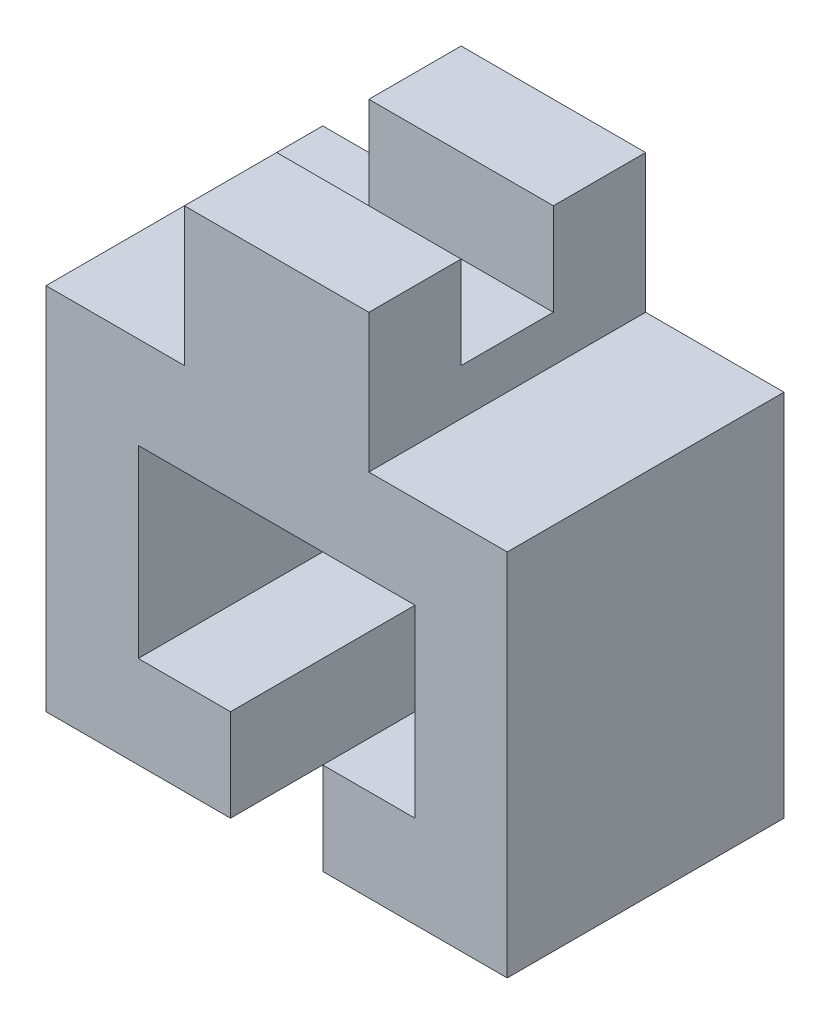
ISO-10303-21;
HEADER;
FILE_DESCRIPTION(('STEP AP214'),'2;1');
FILE_NAME('part.step','',(''),(''),'','','');
FILE_SCHEMA(('AUTOMOTIVE_DESIGN { 1 0 10303 214 1 1 1 1 }'));
ENDSEC;
DATA;
#1=APPLICATION_CONTEXT('core data for automotive mechanical design processes');
#2=APPLICATION_PROTOCOL_DEFINITION('international standard','automotive_design',2000,#1);
#3=PRODUCT_CONTEXT('',#1,'mechanical');
#4=PRODUCT('Part','Part','',(#3));
#5=PRODUCT_RELATED_PRODUCT_CATEGORY('part','',(#4));
#6=PRODUCT_DEFINITION_FORMATION('','',#4);
#7=PRODUCT_DEFINITION_CONTEXT('part definition',#1,'design');
#8=PRODUCT_DEFINITION('design','',#6,#7);
#9=PRODUCT_DEFINITION_SHAPE('','',#8);
#10=(LENGTH_UNIT() NAMED_UNIT(*) SI_UNIT(.MILLI.,.METRE.));
#11=(NAMED_UNIT(*) PLANE_ANGLE_UNIT() SI_UNIT($,.RADIAN.));
#12=(NAMED_UNIT(*) SI_UNIT($,.STERADIAN.) SOLID_ANGLE_UNIT());
#13=UNCERTAINTY_MEASURE_WITH_UNIT(LENGTH_MEASURE(1.E-05),#10,'distance_accuracy_value','');
#14=(GEOMETRIC_REPRESENTATION_CONTEXT(3) GLOBAL_UNCERTAINTY_ASSIGNED_CONTEXT((#13)) GLOBAL_UNIT_ASSIGNED_CONTEXT((#10,
#11,#12)) REPRESENTATION_CONTEXT('',''));
#15=CARTESIAN_POINT('',(0.,0.,0.));
#16=DIRECTION('',(0.,0.,1.));
#17=DIRECTION('',(1.,0.,0.));
#18=AXIS2_PLACEMENT_3D('',#15,#16,#17);
#19=CARTESIAN_POINT('',(15.,55.,30.));
#20=DIRECTION('',(0.,-1.,0.));
#21=DIRECTION('',(0.,0.,-1.));
#22=AXIS2_PLACEMENT_3D('',#19,#20,#21);
#23=PLANE('',#22);
#24=DIRECTION('',(0.,0.,-1.));
#25=VECTOR('',#24,1.);
#26=CARTESIAN_POINT('',(15.,55.,30.));
#27=LINE('',#26,#25);
#28=CARTESIAN_POINT('',(15.,55.,10.));
#29=VERTEX_POINT('',#28);
#30=CARTESIAN_POINT('',(15.,55.,0.));
#31=VERTEX_POINT('',#30);
#32=EDGE_CURVE('E193',#29,#31,#27,.T.);
#33=ORIENTED_EDGE('',*,*,#32,.F.);
#34=DIRECTION('',(-1.,0.,0.));
#35=VECTOR('',#34,1.);
#36=CARTESIAN_POINT('',(15.,55.,10.));
#37=LINE('',#36,#35);
#38=CARTESIAN_POINT('',(35.,55.,10.));
#39=VERTEX_POINT('',#38);
#40=EDGE_CURVE('E346',#39,#29,#37,.T.);
#41=ORIENTED_EDGE('',*,*,#40,.F.);
#42=DIRECTION('',(0.,0.,-1.));
#43=VECTOR('',#42,1.);
#44=CARTESIAN_POINT('',(35.,55.,30.));
#45=LINE('',#44,#43);
#46=CARTESIAN_POINT('',(35.,55.,0.));
#47=VERTEX_POINT('',#46);
#48=EDGE_CURVE('E241',#39,#47,#45,.T.);
#49=ORIENTED_EDGE('',*,*,#48,.T.);
#50=DIRECTION('',(-1.,0.,0.));
#51=VECTOR('',#50,1.);
#52=CARTESIAN_POINT('',(15.,55.,0.));
#53=LINE('',#52,#51);
#54=EDGE_CURVE('E227',#47,#31,#53,.T.);
#55=ORIENTED_EDGE('',*,*,#54,.T.);
#56=EDGE_LOOP('',(#33,#41,#49,#55));
#57=FACE_BOUND('',#56,.T.);
#58=ADVANCED_FACE('F44',(#57),#23,.F.);
#59=CARTESIAN_POINT('',(20.,0.,30.));
#60=DIRECTION('',(0.,1.,0.));
#61=DIRECTION('',(0.,0.,1.));
#62=AXIS2_PLACEMENT_3D('',#59,#60,#61);
#63=PLANE('',#62);
#64=DIRECTION('',(1.,0.,0.));
#65=VECTOR('',#64,1.);
#66=CARTESIAN_POINT('',(20.,0.,0.));
#67=LINE('',#66,#65);
#68=CARTESIAN_POINT('',(0.,0.,0.));
#69=VERTEX_POINT('',#68);
#70=CARTESIAN_POINT('',(20.,0.,0.));
#71=VERTEX_POINT('',#70);
#72=EDGE_CURVE('E201',#69,#71,#67,.T.);
#73=ORIENTED_EDGE('',*,*,#72,.T.);
#74=DIRECTION('',(0.,0.,-1.));
#75=VECTOR('',#74,1.);
#76=CARTESIAN_POINT('',(20.,0.,30.));
#77=LINE('',#76,#75);
#78=CARTESIAN_POINT('',(20.,0.,30.));
#79=VERTEX_POINT('',#78);
#80=EDGE_CURVE('E11',#79,#71,#77,.T.);
#81=ORIENTED_EDGE('',*,*,#80,.F.);
#82=DIRECTION('',(1.,0.,0.));
#83=VECTOR('',#82,1.);
#84=CARTESIAN_POINT('',(20.,0.,30.));
#85=LINE('',#84,#83);
#86=CARTESIAN_POINT('',(0.,0.,30.));
#87=VERTEX_POINT('',#86);
#88=EDGE_CURVE('E240',#87,#79,#85,.T.);
#89=ORIENTED_EDGE('',*,*,#88,.F.);
#90=DIRECTION('',(0.,0.,-1.));
#91=VECTOR('',#90,1.);
#92=CARTESIAN_POINT('',(0.,0.,30.));
#93=LINE('',#92,#91);
#94=EDGE_CURVE('E200',#87,#69,#93,.T.);
#95=ORIENTED_EDGE('',*,*,#94,.T.);
#96=EDGE_LOOP('',(#73,#81,#89,#95));
#97=FACE_BOUND('',#96,.T.);
#98=ADVANCED_FACE('F50',(#97),#63,.F.);
#99=CARTESIAN_POINT('',(20.,10.,30.));
#100=DIRECTION('',(-1.,0.,0.));
#101=DIRECTION('',(0.,0.,1.));
#102=AXIS2_PLACEMENT_3D('',#99,#100,#101);
#103=PLANE('',#102);
#104=DIRECTION('',(0.,1.,0.));
#105=VECTOR('',#104,1.);
#106=CARTESIAN_POINT('',(20.,10.,0.));
#107=LINE('',#106,#105);
#108=CARTESIAN_POINT('',(20.,10.,0.));
#109=VERTEX_POINT('',#108);
#110=EDGE_CURVE('E206',#71,#109,#107,.T.);
#111=ORIENTED_EDGE('',*,*,#110,.T.);
#112=DIRECTION('',(0.,0.,-1.));
#113=VECTOR('',#112,1.);
#114=CARTESIAN_POINT('',(20.,10.,30.));
#115=LINE('',#114,#113);
#116=CARTESIAN_POINT('',(20.,10.,30.));
#117=VERTEX_POINT('',#116);
#118=EDGE_CURVE('E52',#117,#109,#115,.T.);
#119=ORIENTED_EDGE('',*,*,#118,.F.);
#120=DIRECTION('',(0.,1.,0.));
#121=VECTOR('',#120,1.);
#122=CARTESIAN_POINT('',(20.,10.,30.));
#123=LINE('',#122,#121);
#124=EDGE_CURVE('E133',#79,#117,#123,.T.);
#125=ORIENTED_EDGE('',*,*,#124,.F.);
#126=ORIENTED_EDGE('',*,*,#80,.T.);
#127=EDGE_LOOP('',(#111,#119,#125,#126));
#128=FACE_BOUND('',#127,.T.);
#129=ADVANCED_FACE('F369',(#128),#103,.F.);
#130=CARTESIAN_POINT('',(9.99999999999999,10.,30.));
#131=DIRECTION('',(0.,-1.,0.));
#132=DIRECTION('',(0.,0.,-1.));
#133=AXIS2_PLACEMENT_3D('',#130,#131,#132);
#134=PLANE('',#133);
#135=DIRECTION('',(-1.,0.,0.));
#136=VECTOR('',#135,1.);
#137=CARTESIAN_POINT('',(9.99999999999999,10.,0.));
#138=LINE('',#137,#136);
#139=CARTESIAN_POINT('',(9.99999999999999,10.,0.));
#140=VERTEX_POINT('',#139);
#141=EDGE_CURVE('E207',#109,#140,#138,.T.);
#142=ORIENTED_EDGE('',*,*,#141,.T.);
#143=DIRECTION('',(0.,0.,-1.));
#144=VECTOR('',#143,1.);
#145=CARTESIAN_POINT('',(9.99999999999999,10.,30.));
#146=LINE('',#145,#144);
#147=CARTESIAN_POINT('',(9.99999999999999,10.,30.));
#148=VERTEX_POINT('',#147);
#149=EDGE_CURVE('E269',#148,#140,#146,.T.);
#150=ORIENTED_EDGE('',*,*,#149,.F.);
#151=DIRECTION('',(-1.,0.,0.));
#152=VECTOR('',#151,1.);
#153=CARTESIAN_POINT('',(9.99999999999999,10.,30.));
#154=LINE('',#153,#152);
#155=EDGE_CURVE('E279',#117,#148,#154,.T.);
#156=ORIENTED_EDGE('',*,*,#155,.F.);
#157=ORIENTED_EDGE('',*,*,#118,.T.);
#158=EDGE_LOOP('',(#142,#150,#156,#157));
#159=FACE_BOUND('',#158,.T.);
#160=ADVANCED_FACE('F277',(#159),#134,.F.);
#161=CARTESIAN_POINT('',(9.99999999999999,30.,30.));
#162=DIRECTION('',(-1.,0.,0.));
#163=DIRECTION('',(0.,0.,1.));
#164=AXIS2_PLACEMENT_3D('',#161,#162,#163);
#165=PLANE('',#164);
#166=DIRECTION('',(0.,1.,0.));
#167=VECTOR('',#166,1.);
#168=CARTESIAN_POINT('',(9.99999999999999,30.,0.));
#169=LINE('',#168,#167);
#170=CARTESIAN_POINT('',(9.99999999999999,30.,0.));
#171=VERTEX_POINT('',#170);
#172=EDGE_CURVE('E211',#140,#171,#169,.T.);
#173=ORIENTED_EDGE('',*,*,#172,.T.);
#174=DIRECTION('',(0.,0.,-1.));
#175=VECTOR('',#174,1.);
#176=CARTESIAN_POINT('',(9.99999999999999,30.,30.));
#177=LINE('',#176,#175);
#178=CARTESIAN_POINT('',(9.99999999999999,30.,30.));
#179=VERTEX_POINT('',#178);
#180=EDGE_CURVE('E270',#179,#171,#177,.T.);
#181=ORIENTED_EDGE('',*,*,#180,.F.);
#182=DIRECTION('',(0.,1.,0.));
#183=VECTOR('',#182,1.);
#184=CARTESIAN_POINT('',(9.99999999999999,30.,30.));
#185=LINE('',#184,#183);
#186=EDGE_CURVE('E299',#148,#179,#185,.T.);
#187=ORIENTED_EDGE('',*,*,#186,.F.);
#188=ORIENTED_EDGE('',*,*,#149,.T.);
#189=EDGE_LOOP('',(#173,#181,#187,#188));
#190=FACE_BOUND('',#189,.T.);
#191=ADVANCED_FACE('F286',(#190),#165,.F.);
#192=CARTESIAN_POINT('',(40.,30.,30.));
#193=DIRECTION('',(0.,1.,0.));
#194=DIRECTION('',(0.,0.,1.));
#195=AXIS2_PLACEMENT_3D('',#192,#193,#194);
#196=PLANE('',#195);
#197=DIRECTION('',(1.,0.,0.));
#198=VECTOR('',#197,1.);
#199=CARTESIAN_POINT('',(40.,30.,0.));
#200=LINE('',#199,#198);
#201=CARTESIAN_POINT('',(40.,30.,0.));
#202=VERTEX_POINT('',#201);
#203=EDGE_CURVE('E213',#171,#202,#200,.T.);
#204=ORIENTED_EDGE('',*,*,#203,.T.);
#205=DIRECTION('',(0.,0.,-1.));
#206=VECTOR('',#205,1.);
#207=CARTESIAN_POINT('',(40.,30.,30.));
#208=LINE('',#207,#206);
#209=CARTESIAN_POINT('',(40.,30.,30.));
#210=VERTEX_POINT('',#209);
#211=EDGE_CURVE('E262',#210,#202,#208,.T.);
#212=ORIENTED_EDGE('',*,*,#211,.F.);
#213=DIRECTION('',(1.,0.,0.));
#214=VECTOR('',#213,1.);
#215=CARTESIAN_POINT('',(40.,30.,30.));
#216=LINE('',#215,#214);
#217=EDGE_CURVE('E291',#179,#210,#216,.T.);
#218=ORIENTED_EDGE('',*,*,#217,.F.);
#219=ORIENTED_EDGE('',*,*,#180,.T.);
#220=EDGE_LOOP('',(#204,#212,#218,#219));
#221=FACE_BOUND('',#220,.T.);
#222=ADVANCED_FACE('F292',(#221),#196,.F.);
#223=CARTESIAN_POINT('',(40.,10.,30.));
#224=DIRECTION('',(1.,0.,0.));
#225=DIRECTION('',(0.,0.,-1.));
#226=AXIS2_PLACEMENT_3D('',#223,#224,#225);
#227=PLANE('',#226);
#228=DIRECTION('',(0.,-1.,0.));
#229=VECTOR('',#228,1.);
#230=CARTESIAN_POINT('',(40.,10.,0.));
#231=LINE('',#230,#229);
#232=CARTESIAN_POINT('',(40.,10.,0.));
#233=VERTEX_POINT('',#232);
#234=EDGE_CURVE('E214',#202,#233,#231,.T.);
#235=ORIENTED_EDGE('',*,*,#234,.T.);
#236=DIRECTION('',(0.,0.,-1.));
#237=VECTOR('',#236,1.);
#238=CARTESIAN_POINT('',(40.,10.,30.));
#239=LINE('',#238,#237);
#240=CARTESIAN_POINT('',(40.,10.,30.));
#241=VERTEX_POINT('',#240);
#242=EDGE_CURVE('E261',#241,#233,#239,.T.);
#243=ORIENTED_EDGE('',*,*,#242,.F.);
#244=DIRECTION('',(0.,-1.,0.));
#245=VECTOR('',#244,1.);
#246=CARTESIAN_POINT('',(40.,10.,30.));
#247=LINE('',#246,#245);
#248=EDGE_CURVE('E293',#210,#241,#247,.T.);
#249=ORIENTED_EDGE('',*,*,#248,.F.);
#250=ORIENTED_EDGE('',*,*,#211,.T.);
#251=EDGE_LOOP('',(#235,#243,#249,#250));
#252=FACE_BOUND('',#251,.T.);
#253=ADVANCED_FACE('F414',(#252),#227,.F.);
#254=CARTESIAN_POINT('',(30.,10.,30.));
#255=DIRECTION('',(0.,-1.,0.));
#256=DIRECTION('',(0.,0.,-1.));
#257=AXIS2_PLACEMENT_3D('',#254,#255,#256);
#258=PLANE('',#257);
#259=DIRECTION('',(-1.,0.,0.));
#260=VECTOR('',#259,1.);
#261=CARTESIAN_POINT('',(30.,10.,0.));
#262=LINE('',#261,#260);
#263=CARTESIAN_POINT('',(30.,10.,0.));
#264=VERTEX_POINT('',#263);
#265=EDGE_CURVE('E220',#233,#264,#262,.T.);
#266=ORIENTED_EDGE('',*,*,#265,.T.);
#267=DIRECTION('',(0.,0.,-1.));
#268=VECTOR('',#267,1.);
#269=CARTESIAN_POINT('',(30.,10.,30.));
#270=LINE('',#269,#268);
#271=CARTESIAN_POINT('',(30.,10.,30.));
#272=VERTEX_POINT('',#271);
#273=EDGE_CURVE('E256',#272,#264,#270,.T.);
#274=ORIENTED_EDGE('',*,*,#273,.F.);
#275=DIRECTION('',(-1.,0.,0.));
#276=VECTOR('',#275,1.);
#277=CARTESIAN_POINT('',(30.,10.,30.));
#278=LINE('',#277,#276);
#279=EDGE_CURVE('E300',#241,#272,#278,.T.);
#280=ORIENTED_EDGE('',*,*,#279,.F.);
#281=ORIENTED_EDGE('',*,*,#242,.T.);
#282=EDGE_LOOP('',(#266,#274,#280,#281));
#283=FACE_BOUND('',#282,.T.);
#284=ADVANCED_FACE('F406',(#283),#258,.F.);
#285=CARTESIAN_POINT('',(30.,0.,30.));
#286=DIRECTION('',(1.,0.,0.));
#287=DIRECTION('',(0.,0.,-1.));
#288=AXIS2_PLACEMENT_3D('',#285,#286,#287);
#289=PLANE('',#288);
#290=DIRECTION('',(0.,-1.,0.));
#291=VECTOR('',#290,1.);
#292=CARTESIAN_POINT('',(30.,0.,0.));
#293=LINE('',#292,#291);
#294=CARTESIAN_POINT('',(30.,0.,0.));
#295=VERTEX_POINT('',#294);
#296=EDGE_CURVE('E218',#264,#295,#293,.T.);
#297=ORIENTED_EDGE('',*,*,#296,.T.);
#298=DIRECTION('',(0.,0.,-1.));
#299=VECTOR('',#298,1.);
#300=CARTESIAN_POINT('',(30.,0.,30.));
#301=LINE('',#300,#299);
#302=CARTESIAN_POINT('',(30.,0.,30.));
#303=VERTEX_POINT('',#302);
#304=EDGE_CURVE('E254',#303,#295,#301,.T.);
#305=ORIENTED_EDGE('',*,*,#304,.F.);
#306=DIRECTION('',(0.,-1.,0.));
#307=VECTOR('',#306,1.);
#308=CARTESIAN_POINT('',(30.,0.,30.));
#309=LINE('',#308,#307);
#310=EDGE_CURVE('E303',#272,#303,#309,.T.);
#311=ORIENTED_EDGE('',*,*,#310,.F.);
#312=ORIENTED_EDGE('',*,*,#273,.T.);
#313=EDGE_LOOP('',(#297,#305,#311,#312));
#314=FACE_BOUND('',#313,.T.);
#315=ADVANCED_FACE('F401',(#314),#289,.F.);
#316=CARTESIAN_POINT('',(50.,0.,30.));
#317=DIRECTION('',(0.,1.,0.));
#318=DIRECTION('',(0.,0.,1.));
#319=AXIS2_PLACEMENT_3D('',#316,#317,#318);
#320=PLANE('',#319);
#321=DIRECTION('',(1.,0.,0.));
#322=VECTOR('',#321,1.);
#323=CARTESIAN_POINT('',(50.,0.,0.));
#324=LINE('',#323,#322);
#325=CARTESIAN_POINT('',(50.,0.,0.));
#326=VERTEX_POINT('',#325);
#327=EDGE_CURVE('E222',#295,#326,#324,.T.);
#328=ORIENTED_EDGE('',*,*,#327,.T.);
#329=DIRECTION('',(0.,0.,-1.));
#330=VECTOR('',#329,1.);
#331=CARTESIAN_POINT('',(50.,0.,30.));
#332=LINE('',#331,#330);
#333=CARTESIAN_POINT('',(50.,0.,30.));
#334=VERTEX_POINT('',#333);
#335=EDGE_CURVE('E252',#334,#326,#332,.T.);
#336=ORIENTED_EDGE('',*,*,#335,.F.);
#337=DIRECTION('',(1.,0.,0.));
#338=VECTOR('',#337,1.);
#339=CARTESIAN_POINT('',(50.,0.,30.));
#340=LINE('',#339,#338);
#341=EDGE_CURVE('E308',#303,#334,#340,.T.);
#342=ORIENTED_EDGE('',*,*,#341,.F.);
#343=ORIENTED_EDGE('',*,*,#304,.T.);
#344=EDGE_LOOP('',(#328,#336,#342,#343));
#345=FACE_BOUND('',#344,.T.);
#346=ADVANCED_FACE('F398',(#345),#320,.F.);
#347=CARTESIAN_POINT('',(50.,40.,30.));
#348=DIRECTION('',(-1.,0.,0.));
#349=DIRECTION('',(0.,0.,1.));
#350=AXIS2_PLACEMENT_3D('',#347,#348,#349);
#351=PLANE('',#350);
#352=DIRECTION('',(0.,1.,0.));
#353=VECTOR('',#352,1.);
#354=CARTESIAN_POINT('',(50.,40.,0.));
#355=LINE('',#354,#353);
#356=CARTESIAN_POINT('',(50.,40.,0.));
#357=VERTEX_POINT('',#356);
#358=EDGE_CURVE('E224',#326,#357,#355,.T.);
#359=ORIENTED_EDGE('',*,*,#358,.T.);
#360=DIRECTION('',(0.,0.,-1.));
#361=VECTOR('',#360,1.);
#362=CARTESIAN_POINT('',(50.,40.,30.));
#363=LINE('',#362,#361);
#364=CARTESIAN_POINT('',(50.,40.,30.));
#365=VERTEX_POINT('',#364);
#366=EDGE_CURVE('E248',#365,#357,#363,.T.);
#367=ORIENTED_EDGE('',*,*,#366,.F.);
#368=DIRECTION('',(0.,1.,0.));
#369=VECTOR('',#368,1.);
#370=CARTESIAN_POINT('',(50.,40.,30.));
#371=LINE('',#370,#369);
#372=EDGE_CURVE('E306',#334,#365,#371,.T.);
#373=ORIENTED_EDGE('',*,*,#372,.F.);
#374=ORIENTED_EDGE('',*,*,#335,.T.);
#375=EDGE_LOOP('',(#359,#367,#373,#374));
#376=FACE_BOUND('',#375,.T.);
#377=ADVANCED_FACE('F395',(#376),#351,.F.);
#378=CARTESIAN_POINT('',(35.,40.,30.));
#379=DIRECTION('',(0.,-1.,0.));
#380=DIRECTION('',(0.,0.,-1.));
#381=AXIS2_PLACEMENT_3D('',#378,#379,#380);
#382=PLANE('',#381);
#383=DIRECTION('',(-1.,0.,0.));
#384=VECTOR('',#383,1.);
#385=CARTESIAN_POINT('',(35.,40.,0.));
#386=LINE('',#385,#384);
#387=CARTESIAN_POINT('',(35.,40.,0.));
#388=VERTEX_POINT('',#387);
#389=EDGE_CURVE('E223',#357,#388,#386,.T.);
#390=ORIENTED_EDGE('',*,*,#389,.T.);
#391=DIRECTION('',(0.,0.,-1.));
#392=VECTOR('',#391,1.);
#393=CARTESIAN_POINT('',(35.,40.,30.));
#394=LINE('',#393,#392);
#395=CARTESIAN_POINT('',(35.,40.,30.));
#396=VERTEX_POINT('',#395);
#397=EDGE_CURVE('E249',#396,#388,#394,.T.);
#398=ORIENTED_EDGE('',*,*,#397,.F.);
#399=DIRECTION('',(-1.,0.,0.));
#400=VECTOR('',#399,1.);
#401=CARTESIAN_POINT('',(35.,40.,30.));
#402=LINE('',#401,#400);
#403=EDGE_CURVE('E309',#365,#396,#402,.T.);
#404=ORIENTED_EDGE('',*,*,#403,.F.);
#405=ORIENTED_EDGE('',*,*,#366,.T.);
#406=EDGE_LOOP('',(#390,#398,#404,#405));
#407=FACE_BOUND('',#406,.T.);
#408=ADVANCED_FACE('F386',(#407),#382,.F.);
#409=CARTESIAN_POINT('',(35.,55.,30.));
#410=DIRECTION('',(-1.,0.,0.));
#411=DIRECTION('',(0.,0.,1.));
#412=AXIS2_PLACEMENT_3D('',#409,#410,#411);
#413=PLANE('',#412);
#414=ORIENTED_EDGE('',*,*,#48,.F.);
#415=DIRECTION('',(0.,1.,0.));
#416=VECTOR('',#415,1.);
#417=CARTESIAN_POINT('',(35.,45.,10.));
#418=LINE('',#417,#416);
#419=CARTESIAN_POINT('',(35.,45.,10.));
#420=VERTEX_POINT('',#419);
#421=EDGE_CURVE('E347',#420,#39,#418,.T.);
#422=ORIENTED_EDGE('',*,*,#421,.F.);
#423=DIRECTION('',(0.,0.,-1.));
#424=VECTOR('',#423,1.);
#425=CARTESIAN_POINT('',(35.,45.,10.));
#426=LINE('',#425,#424);
#427=CARTESIAN_POINT('',(35.,45.,20.));
#428=VERTEX_POINT('',#427);
#429=EDGE_CURVE('E353',#428,#420,#426,.T.);
#430=ORIENTED_EDGE('',*,*,#429,.F.);
#431=DIRECTION('',(0.,1.,0.));
#432=VECTOR('',#431,1.);
#433=CARTESIAN_POINT('',(35.,45.,20.));
#434=LINE('',#433,#432);
#435=CARTESIAN_POINT('',(35.,55.,20.));
#436=VERTEX_POINT('',#435);
#437=EDGE_CURVE('E322',#428,#436,#434,.T.);
#438=ORIENTED_EDGE('',*,*,#437,.T.);
#439=CARTESIAN_POINT('',(35.,55.,30.));
#440=VERTEX_POINT('',#439);
#441=EDGE_CURVE('E245',#440,#436,#45,.T.);
#442=ORIENTED_EDGE('',*,*,#441,.F.);
#443=DIRECTION('',(0.,1.,0.));
#444=VECTOR('',#443,1.);
#445=CARTESIAN_POINT('',(35.,55.,30.));
#446=LINE('',#445,#444);
#447=EDGE_CURVE('E315',#396,#440,#446,.T.);
#448=ORIENTED_EDGE('',*,*,#447,.F.);
#449=ORIENTED_EDGE('',*,*,#397,.T.);
#450=DIRECTION('',(0.,1.,0.));
#451=VECTOR('',#450,1.);
#452=CARTESIAN_POINT('',(35.,55.,0.));
#453=LINE('',#452,#451);
#454=EDGE_CURVE('E226',#388,#47,#453,.T.);
#455=ORIENTED_EDGE('',*,*,#454,.T.);
#456=EDGE_LOOP('',(#414,#422,#430,#438,#442,#448,#449,#455));
#457=FACE_BOUND('',#456,.T.);
#458=ADVANCED_FACE('F319',(#457),#413,.F.);
#459=ORIENTED_EDGE('',*,*,#441,.T.);
#460=DIRECTION('',(1.,0.,0.));
#461=VECTOR('',#460,1.);
#462=CARTESIAN_POINT('',(35.,55.,20.));
#463=LINE('',#462,#461);
#464=CARTESIAN_POINT('',(15.,55.,20.));
#465=VERTEX_POINT('',#464);
#466=EDGE_CURVE('E329',#465,#436,#463,.T.);
#467=ORIENTED_EDGE('',*,*,#466,.F.);
#468=CARTESIAN_POINT('',(15.,55.,30.));
#469=VERTEX_POINT('',#468);
#470=EDGE_CURVE('E238',#469,#465,#27,.T.);
#471=ORIENTED_EDGE('',*,*,#470,.F.);
#472=DIRECTION('',(-1.,0.,0.));
#473=VECTOR('',#472,1.);
#474=CARTESIAN_POINT('',(15.,55.,30.));
#475=LINE('',#474,#473);
#476=EDGE_CURVE('E182',#440,#469,#475,.T.);
#477=ORIENTED_EDGE('',*,*,#476,.F.);
#478=EDGE_LOOP('',(#459,#467,#471,#477));
#479=FACE_BOUND('',#478,.T.);
#480=ADVANCED_FACE('F330',(#479),#23,.F.);
#481=CARTESIAN_POINT('',(15.,40.,30.));
#482=DIRECTION('',(1.,0.,0.));
#483=DIRECTION('',(0.,0.,-1.));
#484=AXIS2_PLACEMENT_3D('',#481,#482,#483);
#485=PLANE('',#484);
#486=DIRECTION('',(0.,0.,1.));
#487=VECTOR('',#486,1.);
#488=CARTESIAN_POINT('',(15.,45.,10.));
#489=LINE('',#488,#487);
#490=CARTESIAN_POINT('',(15.,45.,10.));
#491=VERTEX_POINT('',#490);
#492=CARTESIAN_POINT('',(15.,45.,20.));
#493=VERTEX_POINT('',#492);
#494=EDGE_CURVE('E671',#491,#493,#489,.T.);
#495=ORIENTED_EDGE('',*,*,#494,.F.);
#496=DIRECTION('',(0.,1.,0.));
#497=VECTOR('',#496,1.);
#498=CARTESIAN_POINT('',(15.,45.,10.));
#499=LINE('',#498,#497);
#500=EDGE_CURVE('E210',#491,#29,#499,.T.);
#501=ORIENTED_EDGE('',*,*,#500,.T.);
#502=ORIENTED_EDGE('',*,*,#32,.T.);
#503=DIRECTION('',(0.,-1.,0.));
#504=VECTOR('',#503,1.);
#505=CARTESIAN_POINT('',(15.,40.,0.));
#506=LINE('',#505,#504);
#507=CARTESIAN_POINT('',(15.,40.,0.));
#508=VERTEX_POINT('',#507);
#509=EDGE_CURVE('E194',#31,#508,#506,.T.);
#510=ORIENTED_EDGE('',*,*,#509,.T.);
#511=DIRECTION('',(0.,0.,-1.));
#512=VECTOR('',#511,1.);
#513=CARTESIAN_POINT('',(15.,40.,30.));
#514=LINE('',#513,#512);
#515=CARTESIAN_POINT('',(15.,40.,30.));
#516=VERTEX_POINT('',#515);
#517=EDGE_CURVE('E186',#516,#508,#514,.T.);
#518=ORIENTED_EDGE('',*,*,#517,.F.);
#519=DIRECTION('',(0.,-1.,0.));
#520=VECTOR('',#519,1.);
#521=CARTESIAN_POINT('',(15.,40.,30.));
#522=LINE('',#521,#520);
#523=EDGE_CURVE('E173',#469,#516,#522,.T.);
#524=ORIENTED_EDGE('',*,*,#523,.F.);
#525=ORIENTED_EDGE('',*,*,#470,.T.);
#526=DIRECTION('',(0.,1.,0.));
#527=VECTOR('',#526,1.);
#528=CARTESIAN_POINT('',(15.,45.,20.));
#529=LINE('',#528,#527);
#530=EDGE_CURVE('E331',#493,#465,#529,.T.);
#531=ORIENTED_EDGE('',*,*,#530,.F.);
#532=EDGE_LOOP('',(#495,#501,#502,#510,#518,#524,#525,#531));
#533=FACE_BOUND('',#532,.T.);
#534=ADVANCED_FACE('F188',(#533),#485,.F.);
#535=CARTESIAN_POINT('',(0.,40.,30.));
#536=DIRECTION('',(0.,-1.,0.));
#537=DIRECTION('',(0.,0.,-1.));
#538=AXIS2_PLACEMENT_3D('',#535,#536,#537);
#539=PLANE('',#538);
#540=DIRECTION('',(-1.,0.,0.));
#541=VECTOR('',#540,1.);
#542=CARTESIAN_POINT('',(0.,40.,0.));
#543=LINE('',#542,#541);
#544=CARTESIAN_POINT('',(0.,40.,0.));
#545=VERTEX_POINT('',#544);
#546=EDGE_CURVE('E233',#508,#545,#543,.T.);
#547=ORIENTED_EDGE('',*,*,#546,.T.);
#548=DIRECTION('',(0.,0.,-1.));
#549=VECTOR('',#548,1.);
#550=CARTESIAN_POINT('',(0.,40.,30.));
#551=LINE('',#550,#549);
#552=CARTESIAN_POINT('',(0.,40.,30.));
#553=VERTEX_POINT('',#552);
#554=EDGE_CURVE('E192',#553,#545,#551,.T.);
#555=ORIENTED_EDGE('',*,*,#554,.F.);
#556=DIRECTION('',(-1.,0.,0.));
#557=VECTOR('',#556,1.);
#558=CARTESIAN_POINT('',(0.,40.,30.));
#559=LINE('',#558,#557);
#560=EDGE_CURVE('E180',#516,#553,#559,.T.);
#561=ORIENTED_EDGE('',*,*,#560,.F.);
#562=ORIENTED_EDGE('',*,*,#517,.T.);
#563=EDGE_LOOP('',(#547,#555,#561,#562));
#564=FACE_BOUND('',#563,.T.);
#565=ADVANCED_FACE('F197',(#564),#539,.F.);
#566=CARTESIAN_POINT('',(0.,0.,30.));
#567=DIRECTION('',(1.,0.,0.));
#568=DIRECTION('',(0.,0.,-1.));
#569=AXIS2_PLACEMENT_3D('',#566,#567,#568);
#570=PLANE('',#569);
#571=DIRECTION('',(0.,-1.,0.));
#572=VECTOR('',#571,1.);
#573=CARTESIAN_POINT('',(0.,0.,0.));
#574=LINE('',#573,#572);
#575=EDGE_CURVE('E127',#545,#69,#574,.T.);
#576=ORIENTED_EDGE('',*,*,#575,.T.);
#577=ORIENTED_EDGE('',*,*,#94,.F.);
#578=DIRECTION('',(0.,-1.,0.));
#579=VECTOR('',#578,1.);
#580=CARTESIAN_POINT('',(0.,0.,30.));
#581=LINE('',#580,#579);
#582=EDGE_CURVE('E68',#553,#87,#581,.T.);
#583=ORIENTED_EDGE('',*,*,#582,.F.);
#584=ORIENTED_EDGE('',*,*,#554,.T.);
#585=EDGE_LOOP('',(#576,#577,#583,#584));
#586=FACE_BOUND('',#585,.T.);
#587=ADVANCED_FACE('F480',(#586),#570,.F.);
#588=CARTESIAN_POINT('',(0.,0.,30.));
#589=DIRECTION('',(0.,0.,-1.));
#590=DIRECTION('',(-1.,0.,0.));
#591=AXIS2_PLACEMENT_3D('',#588,#589,#590);
#592=PLANE('',#591);
#593=ORIENTED_EDGE('',*,*,#88,.T.);
#594=ORIENTED_EDGE('',*,*,#124,.T.);
#595=ORIENTED_EDGE('',*,*,#155,.T.);
#596=ORIENTED_EDGE('',*,*,#186,.T.);
#597=ORIENTED_EDGE('',*,*,#217,.T.);
#598=ORIENTED_EDGE('',*,*,#248,.T.);
#599=ORIENTED_EDGE('',*,*,#279,.T.);
#600=ORIENTED_EDGE('',*,*,#310,.T.);
#601=ORIENTED_EDGE('',*,*,#341,.T.);
#602=ORIENTED_EDGE('',*,*,#372,.T.);
#603=ORIENTED_EDGE('',*,*,#403,.T.);
#604=ORIENTED_EDGE('',*,*,#447,.T.);
#605=ORIENTED_EDGE('',*,*,#476,.T.);
#606=ORIENTED_EDGE('',*,*,#523,.T.);
#607=ORIENTED_EDGE('',*,*,#560,.T.);
#608=ORIENTED_EDGE('',*,*,#582,.T.);
#609=EDGE_LOOP('',(#593,#594,#595,#596,#597,#598,#599,#600,#601,#602,#603,#604,#605,#606,#607,#608));
#610=FACE_BOUND('',#609,.T.);
#611=ADVANCED_FACE('F179',(#610),#592,.F.);
#612=CARTESIAN_POINT('',(0.,0.,0.));
#613=DIRECTION('',(0.,0.,-1.));
#614=DIRECTION('',(-1.,0.,0.));
#615=AXIS2_PLACEMENT_3D('',#612,#613,#614);
#616=PLANE('',#615);
#617=ORIENTED_EDGE('',*,*,#72,.F.);
#618=ORIENTED_EDGE('',*,*,#575,.F.);
#619=ORIENTED_EDGE('',*,*,#546,.F.);
#620=ORIENTED_EDGE('',*,*,#509,.F.);
#621=ORIENTED_EDGE('',*,*,#54,.F.);
#622=ORIENTED_EDGE('',*,*,#454,.F.);
#623=ORIENTED_EDGE('',*,*,#389,.F.);
#624=ORIENTED_EDGE('',*,*,#358,.F.);
#625=ORIENTED_EDGE('',*,*,#327,.F.);
#626=ORIENTED_EDGE('',*,*,#296,.F.);
#627=ORIENTED_EDGE('',*,*,#265,.F.);
#628=ORIENTED_EDGE('',*,*,#234,.F.);
#629=ORIENTED_EDGE('',*,*,#203,.F.);
#630=ORIENTED_EDGE('',*,*,#172,.F.);
#631=ORIENTED_EDGE('',*,*,#141,.F.);
#632=ORIENTED_EDGE('',*,*,#110,.F.);
#633=EDGE_LOOP('',(#617,#618,#619,#620,#621,#622,#623,#624,#625,#626,#627,#628,#629,#630,#631,#632));
#634=FACE_BOUND('',#633,.T.);
#635=ADVANCED_FACE('F281',(#634),#616,.T.);
#636=CARTESIAN_POINT('',(15.,45.,10.));
#637=DIRECTION('',(0.,0.,-1.));
#638=DIRECTION('',(-1.,0.,0.));
#639=AXIS2_PLACEMENT_3D('',#636,#637,#638);
#640=PLANE('',#639);
#641=ORIENTED_EDGE('',*,*,#40,.T.);
#642=ORIENTED_EDGE('',*,*,#500,.F.);
#643=DIRECTION('',(-1.,0.,0.));
#644=VECTOR('',#643,1.);
#645=CARTESIAN_POINT('',(15.,45.,10.));
#646=LINE('',#645,#644);
#647=EDGE_CURVE('E58',#420,#491,#646,.T.);
#648=ORIENTED_EDGE('',*,*,#647,.F.);
#649=ORIENTED_EDGE('',*,*,#421,.T.);
#650=EDGE_LOOP('',(#641,#642,#648,#649));
#651=FACE_BOUND('',#650,.T.);
#652=ADVANCED_FACE('F356',(#651),#640,.F.);
#653=CARTESIAN_POINT('',(35.,45.,20.));
#654=DIRECTION('',(0.,0.,1.));
#655=DIRECTION('',(1.,0.,0.));
#656=AXIS2_PLACEMENT_3D('',#653,#654,#655);
#657=PLANE('',#656);
#658=ORIENTED_EDGE('',*,*,#466,.T.);
#659=ORIENTED_EDGE('',*,*,#437,.F.);
#660=DIRECTION('',(1.,0.,0.));
#661=VECTOR('',#660,1.);
#662=CARTESIAN_POINT('',(35.,45.,20.));
#663=LINE('',#662,#661);
#664=EDGE_CURVE('E355',#493,#428,#663,.T.);
#665=ORIENTED_EDGE('',*,*,#664,.F.);
#666=ORIENTED_EDGE('',*,*,#530,.T.);
#667=EDGE_LOOP('',(#658,#659,#665,#666));
#668=FACE_BOUND('',#667,.T.);
#669=ADVANCED_FACE('F512',(#668),#657,.F.);
#670=CARTESIAN_POINT('',(0.,45.,0.));
#671=DIRECTION('',(0.,-1.,0.));
#672=DIRECTION('',(0.,0.,-1.));
#673=AXIS2_PLACEMENT_3D('',#670,#671,#672);
#674=PLANE('',#673);
#675=ORIENTED_EDGE('',*,*,#494,.T.);
#676=ORIENTED_EDGE('',*,*,#664,.T.);
#677=ORIENTED_EDGE('',*,*,#429,.T.);
#678=ORIENTED_EDGE('',*,*,#647,.T.);
#679=EDGE_LOOP('',(#675,#676,#677,#678));
#680=FACE_BOUND('',#679,.T.);
#681=ADVANCED_FACE('F352',(#680),#674,.F.);
#682=CLOSED_SHELL('',(#58,#98,#129,#160,#191,#222,#253,#284,#315,#346,#377,#408,#458,#480,#534,
#565,#587,#611,#635,#652,#669,#681));
#683=MANIFOLD_SOLID_BREP('B2',#682);
#684=ADVANCED_BREP_SHAPE_REPRESENTATION('',(#18,#683),#14);
#685=SHAPE_DEFINITION_REPRESENTATION(#9,#684);
ENDSEC;
END-ISO-10303-21;
